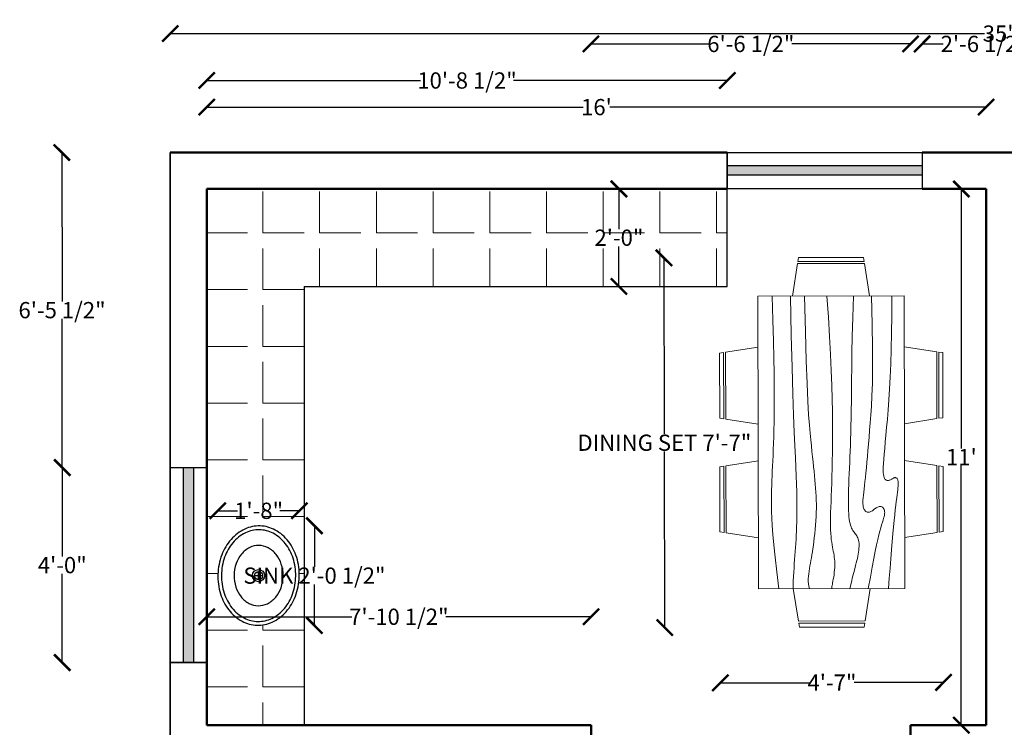
# Model space of a CAD drawing. Units: inches. Extents: x 2466 to 2986, y -30 to 527.
# Tile 3 of 5: x 2469 to 2711, y 353 to 527. Entities that reach past the tile are written whole.
import ezdxf

# ---------------------------------------------------------------- set-up
doc = ezdxf.new("R2010")
doc.units = ezdxf.units.IN
for name, color, linetype, lineweight in [('A-ANNO-DIMS', 2, 'Continuous', 18), ('A-FLOR-CASE', 32, 'Continuous', 25), ('A-FLOR-CASE-PATT', 5, 'Continuous', 13), ('A-FLOR-FIXT', 8, 'Continuous', 25), ('A-GLAZ', 4, 'Continuous', 25), ('A-GLAZ-PATT', 4, 'Continuous', 13), ('C-PROP', 40, 'Continuous', 35), ('furniture', 6, 'Continuous', 18), ('walls', 40, 'Continuous', 50)]:
    doc.layers.add(name, color=color, linetype=linetype, lineweight=lineweight)
doc.styles.get("Standard").update_dxf_attribs({"font": 'arial.ttf'})
doc.dimstyles.get("Standard").update_dxf_attribs({"dimtxt": 4, "dimasz": 4, "dimexe": 0.18, "dimexo": 0.0625, "dimgap": 0.09, "dimtad": 0, "dimtih": 1, "dimtoh": 1, "dimzin": 0, "dimdsep": 46, "dimlunit": 3, "dimtxsty": 'Standard', "dimblk": 'ARCHTICK', "dimcen": 0.09, "dimse1": 1, "dimse2": 1, "dimclrd": 3, "dimclrt": 2, "dimadec": 0, "dimazin": 0, "dimtfac": 1, "dimtofl": 0, "dimtmove": 0, "dimatfit": 3, "dimfxl": 1, "dimtolj": 1, "dimtzin": 0, "dimarcsym": 0})

# ---------------------------------------------------------------- blocks, each defined once
blk = doc.blocks.new('Dining Set - 36 x 72 in.')
for p, q in [((-22, 27.5), (-22.1562, 26.50042)), ((-22, 27.5), (-6, 27.5)), ((-5.8437, 26.49966), (-6, 27.5)), ((6, 27.5), (5.8438, 26.50042)), ((6, 27.5), (22, 27.5)), ((22.1563, 26.49966), (22, 27.5)), ((-22.2343, 26.00059), (-23.4847, 17.99762)), ((-22.2304, 26), (-5.7608, 26)), ((-5.8416, 26.5), (-22.1534, 26.5)), ((-4.5152, 17.99762), (-5.7655, 25.99926)), ((5.7657, 26.00059), (4.5153, 17.99762)), ((5.7696, 26), (22.2392, 26)), ((22.1584, 26.5), (5.8466, 26.5)), ((23.4848, 17.99762), (22.2345, 25.99926)), ((36, 18), (-36, 18)), ((-36, 18), (-36, -18)), ((36, -18), (36, 18)), ((-45.5, 8), (-44.5004, 8.15617)), ((-45.5, 8), (-45.5, -8)), ((-44.5, -8.15843), (-44.5, 8.15338)), ((-44.0006, 8.23428), (-35.9976, 9.48474)), ((-44, 8.23041), (-44, -8.23915)), ((44.0006, 8.23428), (35.9976, 9.48474)), ((44, 8.23041), (44, -8.23915)), ((44.5, -8.15843), (44.5, 8.15338)), ((45.5, 8), (44.5005, 8.15617)), ((45.5, 8), (45.5, -8)), ((-44.4997, -8.15631), (-45.5, -8)), ((-35.9976, -9.48476), (-43.9993, -8.2345)), ((35.9976, -9.48476), (43.9993, -8.2345)), ((44.4997, -8.15631), (45.5, -8)), ((-36, -18), (36, -18)), ((-22.2343, -26.0006), (-23.4847, -17.99762)), ((-4.5152, -17.99762), (-5.7655, -25.99928)), ((5.7657, -26.0006), (4.5153, -17.99762)), ((23.4848, -17.99762), (22.2345, -25.99928)), ((-22.2304, -26), (-5.7608, -26)), ((-22, -27.5), (-22.1562, -26.50044)), ((-5.8416, -26.5), (-22.1534, -26.5)), ((-5.8437, -26.49967), (-6, -27.5)), ((5.7696, -26), (22.2392, -26)), ((6, -27.5), (5.8438, -26.50044)), ((22.1584, -26.5), (5.8466, -26.5)), ((22.1563, -26.49967), (22, -27.5)), ((-22, -27.5), (-6, -27.5)), ((6, -27.5), (22, -27.5))]:
    blk.add_line(p, q)
for points in [[(-36, 15), (-31.1772, 14.97754), (-26.8079, 14.91406), (-22.8538, 14.81543), (-19.276, 14.6875), (-16.0362, 14.53613), (-13.0957, 14.36718), (-10.4159, 14.18652), (-7.9583, 14), (-5.6904, 13.81315), (-3.6035, 13.63021), (-1.6954, 13.45508), (0.0365, 13.29166), (1.5945, 13.14388), (2.9811, 13.01562), (4.1988, 12.9108), (5.25, 12.83333), (6.1393, 12.78613), (6.8802, 12.76823), (7.4883, 12.77767), (7.9792, 12.8125), (8.3685, 12.87077), (8.6719, 12.95052), (8.9049, 13.0498), (9.0833, 13.16666), (9.2205, 13.29899), (9.3216, 13.44401), (9.3895, 13.59879), (9.4271, 13.76041), (9.4373, 13.92594), (9.4232, 14.09245), (9.3875, 14.257), (9.3333, 14.41666), (9.2638, 14.56917), (9.1836, 14.71484), (9.0975, 14.85465), (9.0104, 14.98958), (8.9272, 15.1206), (8.8529, 15.2487), (8.7922, 15.37483), (8.75, 15.5), (8.7305, 15.62467), (8.7344, 15.74739), (8.7617, 15.86621), (8.8125, 15.97916), (8.8867, 16.08431), (8.9844, 16.17968), (9.1055, 16.26334), (9.25, 16.33333), (9.4189, 16.38802), (9.6172, 16.42708), (9.8506, 16.45052), (10.125, 16.45833), (10.4463, 16.45052), (10.8203, 16.42708), (11.2529, 16.38802), (11.75, 16.33333), (12.3184, 16.26318), (12.9694, 16.17838), (13.7151, 16.07991), (14.5677, 15.96875), (15.5395, 15.84586), (16.6426, 15.71224), (17.8893, 15.56884), (19.2917, 15.41666), (20.859, 15.25667), (22.5879, 15.08984), (24.4721, 14.91715), (26.5052, 14.73958), (28.6809, 14.5581), (30.9929, 14.3737), (33.4347, 14.18733), (36, 14)], [(-36, 10), (-28.9766, 10.14274), (-23.1725, 10.20442), (-18.4241, 10.19775), (-14.5677, 10.13541), (-11.4399, 10.03011), (-8.877, 9.89453), (-6.7154, 9.74137), (-4.7917, 9.58333), (-2.9698, 9.43082), (-1.2246, 9.28515), (0.4415, 9.14534), (2.026, 9.01041), (3.5266, 8.87939), (4.9408, 8.7513), (6.266, 8.62516), (7.5, 8.5), (8.6411, 8.37549), (9.6914, 8.2539), (10.6538, 8.13818), (11.5312, 8.03125), (12.3267, 7.93603), (13.043, 7.85547), (13.6831, 7.79248), (14.25, 7.75), (14.7471, 7.7303), (15.1797, 7.73307), (15.5537, 7.75732), (15.875, 7.80208), (16.1494, 7.86637), (16.3828, 7.94922), (16.5811, 8.04964), (16.75, 8.16666), (16.8944, 8.29915), (17.0143, 8.44531), (17.1089, 8.60319), (17.1771, 8.77083), (17.218, 8.94629), (17.2305, 9.1276), (17.2137, 9.31282), (17.1667, 9.5), (17.0895, 9.6875), (16.987, 9.875), (16.8649, 10.0625), (16.7292, 10.25), (16.5856, 10.4375), (16.4401, 10.625), (16.2985, 10.8125), (16.1667, 11), (16.05, 11.18733), (15.9518, 11.3737), (15.8752, 11.5581), (15.8229, 11.73958), (15.798, 11.91715), (15.8034, 12.08984), (15.842, 12.25667), (15.9167, 12.41666), (16.0295, 12.56836), (16.1784, 12.70833), (16.3605, 12.83268), (16.5729, 12.9375), (16.8127, 13.01888), (17.0768, 13.07291), (17.3625, 13.0957), (17.6667, 13.08333), (17.9894, 13.03312), (18.3418, 12.94726), (18.7382, 12.82918), (19.1927, 12.68229), (19.7195, 12.51001), (20.3327, 12.31575), (21.0465, 12.10294), (21.875, 11.875), (22.8357, 11.63354), (23.959, 11.37304), (25.2786, 11.08618), (26.8282, 10.76562), (28.6414, 10.40405), (30.752, 9.99414), (33.1936, 9.52856), (36, 9)], [(-36, 5.5), (-30.7157, 5.3348), (-26.069, 5.20963), (-21.9946, 5.11767), (-18.4271, 5.05208), (-15.3009, 5.00602), (-12.5508, 4.97265), (-10.1112, 4.94515), (-7.9167, 4.91666), (-5.909, 4.88167), (-4.0586, 4.83984), (-2.3429, 4.79215), (-0.7396, 4.73958), (0.7739, 4.6831), (2.22, 4.6237), (3.6213, 4.56233), (5, 4.5), (6.373, 4.43782), (7.7344, 4.3776), (9.0723, 4.32129), (10.375, 4.27083), (11.6309, 4.22819), (12.8281, 4.19531), (13.9551, 4.17415), (15, 4.16666), (15.954, 4.17448), (16.819, 4.19791), (17.6001, 4.23698), (18.3021, 4.29166), (18.9299, 4.36198), (19.4883, 4.44791), (19.9823, 4.54948), (20.4167, 4.66666), (20.7969, 4.79899), (21.1302, 4.94401), (21.4245, 5.09879), (21.6875, 5.26041), (21.9271, 5.42594), (22.1511, 5.59245), (22.3672, 5.757), (22.5834, 5.91666), (22.8065, 6.06868), (23.0404, 6.21093), (23.2879, 6.34147), (23.5521, 6.45833), (23.8358, 6.55957), (24.142, 6.64323), (24.4735, 6.70735), (24.8334, 6.75), (25.2235, 6.76969), (25.642, 6.76692), (26.0858, 6.74267), (26.5521, 6.69791), (27.0379, 6.63362), (27.5404, 6.55078), (28.0565, 6.45036), (28.5834, 6.33333), (29.1242, 6.19987), (29.7071, 6.04687), (30.3661, 5.87044), (31.1354, 5.66666), (32.0493, 5.43164), (33.142, 5.16146), (34.4475, 4.85221), (36, 4.5)], [(-36, -1), (-30.7915, -0.6591), (-26.0195, -0.38216), (-21.6519, -0.16284), (-17.6563, 0.00521), (-14.0005, 0.12833), (-10.6523, 0.21289), (-7.5796, 0.26522), (-4.75, 0.29166), (-2.134, 0.29793), (0.2878, 0.28711), (2.5317, 0.26163), (4.6146, 0.22396), (6.5529, 0.17651), (8.3633, 0.12174), (10.0623, 0.06209), (11.6667, 0), (13.1899, -0.06201), (14.6341, -0.1211), (15.9982, -0.17432), (17.2813, -0.21875), (18.4823, -0.25147), (19.6003, -0.26953), (20.6343, -0.27002), (21.5834, -0.25), (22.4481, -0.20768), (23.2357, -0.14584), (23.9549, -0.06836), (24.6146, 0.02083), (25.2235, 0.11784), (25.7904, 0.21875), (26.3241, 0.31966), (26.8334, 0.41666), (27.3265, 0.50618), (27.8099, 0.58593), (28.2894, 0.65397), (28.7709, 0.70833), (29.2601, 0.74707), (29.763, 0.76823), (30.2855, 0.76985), (30.8334, 0.75), (31.4088, 0.70784), (31.9994, 0.64713), (32.589, 0.57275), (33.1615, 0.48958), (33.7008, 0.4025), (34.1908, 0.3164), (34.6153, 0.23616), (34.9584, 0.16666), (35.2099, 0.11165), (35.3848, 0.07031), (35.504, 0.04069), (35.5886, 0.02083), (35.6594, 0.00879), (35.7377, 0.0026), (35.8442, 0.00032), (36, 0)], [(-36, -6.5), (-27.1843, -6.31267), (-20.084, -6.1263), (-14.469, -5.9419), (-10.1094, -5.76042), (-6.7752, -5.58285), (-4.2363, -5.41016), (-2.2629, -5.24333), (-0.625, -5.08334), (0.8708, -4.93099), (2.2715, -4.78646), (3.5872, -4.64974), (4.8281, -4.52084), (6.0046, -4.39974), (7.127, -4.28646), (8.2053, -4.18099), (9.25, -4.08334), (10.2705, -3.99382), (11.2734, -3.91407), (12.2647, -3.84603), (13.25, -3.79167), (14.2354, -3.75293), (15.2266, -3.73177), (16.2295, -3.73015), (17.25, -3.75), (18.2912, -3.79248), (19.3451, -3.85547), (20.4009, -3.93604), (21.4479, -4.03125), (22.4754, -4.13819), (23.4727, -4.25391), (24.4289, -4.37549), (25.3334, -4.5), (26.1785, -4.62492), (26.9694, -4.74935), (27.7145, -4.87281), (28.4219, -4.99479), (29.1, -5.11483), (29.7572, -5.23242), (30.4016, -5.34709), (31.0417, -5.45834), (31.6837, -5.56437), (32.3262, -5.65821), (32.9658, -5.73153), (33.599, -5.77604), (34.2224, -5.78345), (34.8327, -5.74545), (35.4264, -5.65373), (36, -5.5)], [(-36, -10), (-26.4022, -9.81299), (-18.4675, -9.62891), (-11.9839, -9.45069), (-6.7396, -9.28125), (-2.5226, -9.12354), (0.8789, -8.98047), (3.6769, -8.85498), (6.0833, -8.75), (8.2767, -8.66765), (10.3021, -8.60677), (12.1712, -8.56543), (13.8958, -8.54167), (15.4876, -8.53353), (16.9583, -8.53907), (18.3197, -8.55632), (19.5834, -8.58334), (20.7616, -8.61841), (21.8685, -8.66081), (22.9188, -8.71004), (23.9271, -8.76563), (24.9081, -8.82707), (25.8763, -8.89388), (26.8465, -8.96558), (27.8334, -9.04167), (28.8474, -9.12118), (29.8828, -9.20117), (30.93, -9.27824), (31.9792, -9.34896), (33.0205, -9.40991), (34.0443, -9.45768), (35.0407, -9.48885), (36, -9.5)], [(-36, -14.5), (-30.0881, -14.33513), (-25.0332, -14.21224), (-20.7312, -14.12647), (-17.0781, -14.07292), (-13.97, -14.04671), (-11.3027, -14.04297), (-8.9724, -14.05681), (-6.875, -14.08334), (-4.9224, -14.11833), (-3.0905, -14.16016), (-1.3709, -14.20785), (0.2448, -14.26042), (1.7647, -14.3169), (3.1973, -14.3763), (4.5507, -14.43767), (5.8333, -14.5), (7.0554, -14.5621), (8.235, -14.62175), (9.3922, -14.67652), (10.5469, -14.72396), (11.7192, -14.76164), (12.929, -14.78711), (14.1965, -14.79794), (15.5417, -14.79167), (16.9933, -14.76424), (18.6152, -14.70508), (20.4804, -14.60197), (22.6615, -14.44271), (25.2312, -14.21509), (28.2624, -13.9069), (31.8277, -13.50594), (36, -13)]]:
    blk.add_lwpolyline(points)
blk = doc.blocks.new('Sink - Oval top')
for p, q in [((-1, 0), (1, 0)), ((0, 1), (0, -1))]:
    blk.add_line(p, q)
for points in [[(-12.23, 0.39, 0.117634), (-11.46, -3.36, 0.104469), (-8.88, -6.8, 0.090016), (-5.08, -9.07, 0.08192), (-0.32, -10.02, 0.08192), (4.49, -9.38, 0.090016), (8.42, -7.36, 0.104469), (11.22, -4.09, 0.117634), (12.23, -0.39, 0.117634), (11.46, 3.36, 0.104469), (8.88, 6.8, 0.090016), (5.08, 9.07, 0.08192), (0.32, 10.02, 0.08192), (-4.49, 9.38, 0.090016), (-8.42, 7.36, 0.104469), (-11.22, 4.09, 0.117634)], [(-11.29, 0.16, 0.118622), (-10.52, -3.25, 0.104678), (-8.07, -6.36, 0.089562), (-4.54, -8.37, 0.081185), (-0.13, -9.15, 0.081185), (4.3, -8.49, 0.089562), (7.89, -6.58, 0.104678), (10.42, -3.55, 0.118622), (11.29, -0.16, 0.118622), (10.52, 3.25, 0.104678), (8.07, 6.36, 0.089562), (4.54, 8.37, 0.081185), (0.13, 9.15, 0.081185), (-4.3, 8.49, 0.089562), (-7.89, 6.58, 0.104678), (-10.42, 3.55, 0.118622)], [(-7.42, 0.08, 0.118283), (-6.91, -2.17, 0.104607), (-5.29, -4.21, 0.089718), (-2.97, -5.53, 0.081436), (-0.07, -6.04, 0.081436), (2.84, -5.59, 0.089718), (5.2, -4.33, 0.104607), (6.86, -2.32, 0.118283), (7.42, -0.08, 0.118283), (6.91, 2.17, 0.104607), (5.29, 4.21, 0.089718), (2.97, 5.53, 0.081436), (0.07, 6.04, 0.081436), (-2.84, 5.59, 0.089718), (-5.2, 4.33, 0.104607), (-6.86, 2.32, 0.118283)]]:
    blk.add_lwpolyline(points, format="xyb", close=True)
for radius in [1.5, 1]:
    blk.add_circle((0, 0), radius)
blk = doc.blocks.new('_ArchTick')
at = {"color": 0, "linetype": 'ByBlock', "const_width": 0.15}
blk.add_lwpolyline([(-0.5, -0.5), (0.5, 0.5)], dxfattribs=at)
blk = doc.blocks.new('*D21')
at = {"layer": 'A-ANNO-DIMS', "color": 0, "lineweight": -2, "transparency": 16777216}
for p, q in [((2505.73, 524.05), (2706.38, 524.05)), ((2928.73, 524.05), (2728.07, 524.05))]:
    blk.add_line(p, q, dxfattribs=at)
at = {"layer": 'Defpoints', "color": 0, "transparency": 16777216}
for p in [(2928.73, 524.05), (2505.73, 494.8), (2928.73, 494.8)]:
    blk.add_point(p, dxfattribs=at)
at = {"layer": 'A-ANNO-DIMS', "color": 0, "lineweight": -2, "transparency": 16777216, "xscale": 4, "yscale": 4, "zscale": 4, "rotation": 180}
blk.add_blockref('_ArchTick', (2505.73, 524.05), dxfattribs=at)
at = {"layer": 'A-ANNO-DIMS', "color": 0, "lineweight": -2, "transparency": 16777216, "xscale": 4, "yscale": 4, "zscale": 4}
blk.add_blockref('_ArchTick', (2928.73, 524.05), dxfattribs=at)
at = {"layer": 'A-ANNO-DIMS', "color": 0, "transparency": 16777216, "insert": (2717.23, 524.05), "char_height": 4, "attachment_point": 5}
blk.add_mtext('\\A1;35\'-3.00"', dxfattribs=at)
blk = doc.blocks.new('*D23')
at = {"layer": 'A-ANNO-DIMS', "color": 0, "lineweight": -2, "transparency": 16777216}
for p, q in [((2514.73, 505.95), (2607.43, 505.95)), ((2706.73, 505.95), (2614.02, 505.95))]:
    blk.add_line(p, q, dxfattribs=at)
at = {"layer": 'Defpoints', "color": 0, "transparency": 16777216}
for p in [(2706.73, 505.95), (2514.73, 485.8), (2706.73, 485.8)]:
    blk.add_point(p, dxfattribs=at)
at = {"layer": 'A-ANNO-DIMS', "color": 0, "lineweight": -2, "transparency": 16777216, "xscale": 4, "yscale": 4, "zscale": 4, "rotation": 180}
blk.add_blockref('_ArchTick', (2514.73, 505.95), dxfattribs=at)
at = {"layer": 'A-ANNO-DIMS', "color": 0, "lineweight": -2, "transparency": 16777216, "xscale": 4, "yscale": 4, "zscale": 4}
blk.add_blockref('_ArchTick', (2706.73, 505.95), dxfattribs=at)
at = {"layer": 'A-ANNO-DIMS', "color": 0, "transparency": 16777216, "insert": (2610.73, 505.95), "char_height": 4, "attachment_point": 5}
blk.add_mtext("\\A1;16'", dxfattribs=at)
blk = doc.blocks.new('*D25')
at = {"layer": 'A-ANNO-DIMS', "color": 0, "lineweight": -2, "transparency": 16777216}
for p, q in [((2700.63, 485.8), (2700.63, 421.89)), ((2700.63, 353.8), (2700.63, 417.7))]:
    blk.add_line(p, q, dxfattribs=at)
at = {"layer": 'Defpoints', "color": 0, "transparency": 16777216}
for p in [(2706.73, 485.8), (2700.63, 353.8), (2706.73, 353.8)]:
    blk.add_point(p, dxfattribs=at)
at = {"layer": 'A-ANNO-DIMS', "color": 0, "lineweight": -2, "transparency": 16777216, "xscale": 4, "yscale": 4, "zscale": 4}
for p, rotation in [((2700.63, 485.8), 90), ((2700.63, 353.8), 270)]:
    blk.add_blockref('_ArchTick', p, dxfattribs=dict(at, rotation=rotation))
at = {"layer": 'A-ANNO-DIMS', "color": 0, "transparency": 16777216, "insert": (2700.63, 419.8), "char_height": 4, "attachment_point": 5}
blk.add_mtext("\\A1;11'", dxfattribs=at)
blk = doc.blocks.new('WIN-48IN')
h = blk.add_hatch(color=256)
h.dxf.hatch_style = 1
h.paths.add_polyline_path([(0, 5.81), (0, 3.39), (48, 3.39), (48, 5.81)])
for p, q in [((0, 9), (0, 0)), ((48, 9), (48, 0))]:
    blk.add_line(p, q)
for points in [[(0, 9), (48, 9), (48, 0), (0, 0)], [(0, 5.81), (48, 5.81), (48, 3.39), (0, 3.39)]]:
    blk.add_lwpolyline(points, close=True)
blk = doc.blocks.new('*D53')
at = {"layer": 'A-ANNO-DIMS', "color": 3, "lineweight": -2, "transparency": 16777216}
for p, q in [((2627.36, 468.84), (2627.46, 425.5)), ((2627.58, 377.84), (2627.47, 421.18))]:
    blk.add_line(p, q, dxfattribs=at)
at = {"layer": 'Defpoints', "color": 0, "transparency": 16777216}
for p in [(2641.01, 468.87), (2627.58, 377.84), (2641.23, 377.87)]:
    blk.add_point(p, dxfattribs=at)
at = {"layer": 'A-ANNO-DIMS', "color": 3, "lineweight": -2, "transparency": 16777216, "xscale": 4, "yscale": 4, "zscale": 4}
for p, rotation in [((2627.36, 468.84), 90.1373256303258), ((2627.58, 377.84), 270.1373256303258)]:
    blk.add_blockref('_ArchTick', p, dxfattribs=dict(at, rotation=rotation))
at = {"layer": 'A-ANNO-DIMS', "color": 2, "transparency": 16777216, "insert": (2627.47, 423.34), "char_height": 4, "attachment_point": 5}
blk.add_mtext('\\A1;DINING SET 7\'-7"', dxfattribs=at)
blk = doc.blocks.new('*D54')
at = {"layer": 'A-ANNO-DIMS', "color": 3, "lineweight": -2, "transparency": 16777216}
for p, q in [((2641.26, 364.22), (2663.27, 364.27)), ((2696.26, 364.35), (2674.25, 364.3))]:
    blk.add_line(p, q, dxfattribs=at)
at = {"layer": 'Defpoints', "color": 0, "transparency": 16777216}
for p in [(2641.23, 377.87), (2696.23, 378), (2696.26, 364.35)]:
    blk.add_point(p, dxfattribs=at)
at = {"layer": 'A-ANNO-DIMS', "color": 3, "lineweight": -2, "transparency": 16777216, "xscale": 4, "yscale": 4, "zscale": 4}
for p, rotation in [((2641.26, 364.22), 180.1373256303259), ((2696.26, 364.35), 0.1373256303258501)]:
    blk.add_blockref('_ArchTick', p, dxfattribs=dict(at, rotation=rotation))
at = {"layer": 'A-ANNO-DIMS', "color": 2, "transparency": 16777216, "insert": (2668.76, 364.29), "char_height": 4, "attachment_point": 5}
blk.add_mtext('\\A1;4\'-7"', dxfattribs=at)
blk = doc.blocks.new('*D59')
at = {"layer": 'A-ANNO-DIMS', "color": 3, "lineweight": -2, "transparency": 16777216}
for p, q in [((2541.26, 402.9), (2541.26, 392.78)), ((2541.26, 378.35), (2541.26, 388.46))]:
    blk.add_line(p, q, dxfattribs=at)
at = {"layer": 'Defpoints', "color": 0, "transparency": 16777216}
for p in [(2537.57, 402.9), (2541.26, 402.9), (2537.57, 378.35)]:
    blk.add_point(p, dxfattribs=at)
at = {"layer": 'A-ANNO-DIMS', "color": 3, "lineweight": -2, "transparency": 16777216, "xscale": 4, "yscale": 4, "zscale": 4}
for p, rotation in [((2541.26, 402.9), 90), ((2541.26, 378.35), 270)]:
    blk.add_blockref('_ArchTick', p, dxfattribs=dict(at, rotation=rotation))
at = {"layer": 'A-ANNO-DIMS', "color": 2, "transparency": 16777216, "insert": (2541.26, 390.62), "char_height": 4, "attachment_point": 5}
blk.add_mtext('\\A1;SINK 2\'-0 1/2"', dxfattribs=at)
blk = doc.blocks.new('*D60')
at = {"layer": 'A-ANNO-DIMS', "color": 3, "lineweight": -2, "transparency": 16777216}
for p, q in [((2517.44, 406.58), (2522.29, 406.58)), ((2537.57, 406.58), (2532.72, 406.58))]:
    blk.add_line(p, q, dxfattribs=at)
at = {"layer": 'Defpoints', "color": 0, "transparency": 16777216}
for p in [(2517.44, 406.58), (2517.44, 402.9), (2537.57, 402.9)]:
    blk.add_point(p, dxfattribs=at)
at = {"layer": 'A-ANNO-DIMS', "color": 3, "lineweight": -2, "transparency": 16777216, "xscale": 4, "yscale": 4, "zscale": 4, "rotation": 180}
blk.add_blockref('_ArchTick', (2517.44, 406.58), dxfattribs=at)
at = {"layer": 'A-ANNO-DIMS', "color": 3, "lineweight": -2, "transparency": 16777216, "xscale": 4, "yscale": 4, "zscale": 4}
blk.add_blockref('_ArchTick', (2537.57, 406.58), dxfattribs=at)
at = {"layer": 'A-ANNO-DIMS', "color": 2, "transparency": 16777216, "insert": (2527.51, 406.58), "char_height": 4, "attachment_point": 5}
blk.add_mtext('\\A1;1\'-8"', dxfattribs=at)
blk = doc.blocks.new('*D62')
at = {"layer": 'A-ANNO-DIMS', "color": 3, "lineweight": -2, "transparency": 16777216}
for p, q in [((2609.4, 521.5), (2638.69, 521.5)), ((2688.14, 521.5), (2658.85, 521.5))]:
    blk.add_line(p, q, dxfattribs=at)
at = {"layer": 'Defpoints', "color": 0, "transparency": 16777216}
for p in [(2688.14, 521.5), (2609.4, 353.8), (2688.14, 353.8)]:
    blk.add_point(p, dxfattribs=at)
at = {"layer": 'A-ANNO-DIMS', "color": 3, "lineweight": -2, "transparency": 16777216, "xscale": 4, "yscale": 4, "zscale": 4, "rotation": 180}
blk.add_blockref('_ArchTick', (2609.4, 521.5), dxfattribs=at)
at = {"layer": 'A-ANNO-DIMS', "color": 3, "lineweight": -2, "transparency": 16777216, "xscale": 4, "yscale": 4, "zscale": 4}
blk.add_blockref('_ArchTick', (2688.14, 521.5), dxfattribs=at)
at = {"layer": 'A-ANNO-DIMS', "color": 2, "transparency": 16777216, "insert": (2648.77, 521.5), "char_height": 4, "attachment_point": 5}
blk.add_mtext('\\A1;6\'-6 1/2"', dxfattribs=at)
blk = doc.blocks.new('*D69')
at = {"layer": 'A-ANNO-DIMS', "color": 3, "lineweight": -2, "transparency": 16777216}
for p, q in [((2616.28, 485.8), (2616.28, 475.93)), ((2616.28, 461.8), (2616.28, 471.66))]:
    blk.add_line(p, q, dxfattribs=at)
at = {"layer": 'Defpoints', "color": 0, "transparency": 16777216}
for p in [(2616.28, 485.8), (2642.98, 485.8), (2642.98, 461.8)]:
    blk.add_point(p, dxfattribs=at)
at = {"layer": 'A-ANNO-DIMS', "color": 3, "lineweight": -2, "transparency": 16777216, "xscale": 4, "yscale": 4, "zscale": 4}
for p, rotation in [((2616.28, 485.8), 90), ((2616.28, 461.8), 270)]:
    blk.add_blockref('_ArchTick', p, dxfattribs=dict(at, rotation=rotation))
at = {"layer": 'A-ANNO-DIMS', "color": 2, "transparency": 16777216, "insert": (2616.28, 473.8), "char_height": 4, "attachment_point": 5}
blk.add_mtext('\\A1;2\'-0"', dxfattribs=at)
blk = doc.blocks.new('*D72')
at = {"layer": 'A-ANNO-DIMS', "color": 3, "lineweight": -2, "transparency": 16777216}
for p, q in [((2514.73, 512.5), (2567.42, 512.5)), ((2642.98, 512.5), (2590.28, 512.5))]:
    blk.add_line(p, q, dxfattribs=at)
at = {"layer": 'Defpoints', "color": 0, "transparency": 16777216}
for p in [(2642.98, 512.5), (2514.73, 485.8), (2642.98, 485.8)]:
    blk.add_point(p, dxfattribs=at)
at = {"layer": 'A-ANNO-DIMS', "color": 3, "lineweight": -2, "transparency": 16777216, "xscale": 4, "yscale": 4, "zscale": 4, "rotation": 180}
blk.add_blockref('_ArchTick', (2514.73, 512.5), dxfattribs=at)
at = {"layer": 'A-ANNO-DIMS', "color": 3, "lineweight": -2, "transparency": 16777216, "xscale": 4, "yscale": 4, "zscale": 4}
blk.add_blockref('_ArchTick', (2642.98, 512.5), dxfattribs=at)
at = {"layer": 'A-ANNO-DIMS', "color": 2, "transparency": 16777216, "insert": (2578.85, 512.5), "char_height": 4, "attachment_point": 5}
blk.add_mtext('\\A1;10\'-8 1/2"', dxfattribs=at)
blk = doc.blocks.new('*D73')
at = {"layer": 'A-ANNO-DIMS', "color": 3, "lineweight": -2, "transparency": 16777216}
for p, q in [((2690.98, 521.5), (2696.18, 521.5)), ((2721.59, 521.5), (2716.38, 521.5))]:
    blk.add_line(p, q, dxfattribs=at)
at = {"layer": 'Defpoints', "color": 0, "transparency": 16777216}
for p in [(2721.59, 521.5), (2690.98, 494.8), (2721.59, 494.8)]:
    blk.add_point(p, dxfattribs=at)
at = {"layer": 'A-ANNO-DIMS', "color": 3, "lineweight": -2, "transparency": 16777216, "xscale": 4, "yscale": 4, "zscale": 4, "rotation": 180}
blk.add_blockref('_ArchTick', (2690.98, 521.5), dxfattribs=at)
at = {"layer": 'A-ANNO-DIMS', "color": 3, "lineweight": -2, "transparency": 16777216, "xscale": 4, "yscale": 4, "zscale": 4}
blk.add_blockref('_ArchTick', (2721.59, 521.5), dxfattribs=at)
at = {"layer": 'A-ANNO-DIMS', "color": 2, "transparency": 16777216, "insert": (2706.28, 521.5), "char_height": 4, "attachment_point": 5}
blk.add_mtext('\\A1;2\'-6 1/2"', dxfattribs=at)
blk = doc.blocks.new('*D74')
at = {"layer": 'A-ANNO-DIMS', "color": 3, "lineweight": -2, "transparency": 16777216}
for p, q in [((2479.03, 494.76), (2479.07, 458.13)), ((2479.13, 417.18), (2479.08, 453.81))]:
    blk.add_line(p, q, dxfattribs=at)
at = {"layer": 'Defpoints', "color": 0, "transparency": 16777216}
for p in [(2479.03, 494.76), (2505.73, 494.8), (2505.83, 417.21)]:
    blk.add_point(p, dxfattribs=at)
at = {"layer": 'A-ANNO-DIMS', "color": 3, "lineweight": -2, "transparency": 16777216, "xscale": 4, "yscale": 4, "zscale": 4}
for p, rotation in [((2479.03, 494.76), 90.07540096896105), ((2479.13, 417.18), 270.075400968961)]:
    blk.add_blockref('_ArchTick', p, dxfattribs=dict(at, rotation=rotation))
at = {"layer": 'A-ANNO-DIMS', "color": 2, "transparency": 16777216, "insert": (2479.08, 455.97), "char_height": 4, "attachment_point": 5}
blk.add_mtext('\\A1;6\'-5 1/2"', dxfattribs=at)
blk = doc.blocks.new('*D82')
at = {"layer": 'A-ANNO-DIMS', "color": 3, "lineweight": -2, "transparency": 16777216}
for p, q in [((2479.13, 417.21), (2479.13, 395.34)), ((2479.13, 369.21), (2479.13, 391.08))]:
    blk.add_line(p, q, dxfattribs=at)
at = {"layer": 'Defpoints', "color": 0, "transparency": 16777216}
for p in [(2479.13, 417.21), (2505.83, 417.21), (2505.83, 369.21)]:
    blk.add_point(p, dxfattribs=at)
at = {"layer": 'A-ANNO-DIMS', "color": 3, "lineweight": -2, "transparency": 16777216, "xscale": 4, "yscale": 4, "zscale": 4}
for p, rotation in [((2479.13, 417.21), 90), ((2479.13, 369.21), 270)]:
    blk.add_blockref('_ArchTick', p, dxfattribs=dict(at, rotation=rotation))
at = {"layer": 'A-ANNO-DIMS', "color": 2, "transparency": 16777216, "insert": (2479.13, 393.21), "char_height": 4, "attachment_point": 5}
blk.add_mtext('\\A1;4\'-0"', dxfattribs=at)
blk = doc.blocks.new('*D84')
at = {"layer": 'A-ANNO-DIMS', "color": 3, "lineweight": -2, "transparency": 16777216}
for p, q in [((2514.73, 380.5), (2550.46, 380.5)), ((2609.4, 380.5), (2573.67, 380.5))]:
    blk.add_line(p, q, dxfattribs=at)
at = {"layer": 'Defpoints', "color": 0, "transparency": 16777216}
for p in [(2609.4, 380.5), (2514.73, 353.8), (2609.4, 353.8)]:
    blk.add_point(p, dxfattribs=at)
at = {"layer": 'A-ANNO-DIMS', "color": 3, "lineweight": -2, "transparency": 16777216, "xscale": 4, "yscale": 4, "zscale": 4, "rotation": 180}
blk.add_blockref('_ArchTick', (2514.73, 380.5), dxfattribs=at)
at = {"layer": 'A-ANNO-DIMS', "color": 3, "lineweight": -2, "transparency": 16777216, "xscale": 4, "yscale": 4, "zscale": 4}
blk.add_blockref('_ArchTick', (2609.4, 380.5), dxfattribs=at)
at = {"layer": 'A-ANNO-DIMS', "color": 2, "transparency": 16777216, "insert": (2562.06, 380.5), "char_height": 4, "attachment_point": 5}
blk.add_mtext('\\A1;7\'-10 1/2"', dxfattribs=at)

msp = doc.modelspace()

# ---------------------------------------------------------------- hatches: boundary and pattern name
at = {"layer": 'A-FLOR-CASE-PATT'}
h = msp.add_hatch(dxfattribs=at)
h.set_pattern_fill('ANGLE', color=256, scale=2)
h.set_pattern_definition([(0, (0, 0), (0, 13.97), [10.16, -3.81]), (90, (0, 0), (-13.97, 9e-16), [10.16, -3.81])])
h.paths.add_polyline_path([(2642.976, 485.795), (2514.725, 485.795), (2514.725, 417.211), (2514.828, 417.211), (2514.828, 369.211), (2514.725, 353.795), (2538.725, 353.795), (2538.725, 461.795), (2642.976, 461.795)])
h.paths.add_polyline_path([(2527.9, 402.857, -0.1176343), (2531.599, 401.847, -0.1044693), (2534.867, 399.045, -0.0900158), (2536.886, 395.111, -0.0819199), (2537.521, 390.3, -0.0819199), (2536.578, 385.54, -0.0900158), (2534.309, 381.744, -0.1044693), (2530.867, 379.158, -0.1176343), (2527.111, 378.389, -0.1176343), (2523.413, 379.398, -0.1044693), (2520.145, 382.2, -0.0900158), (2518.125, 386.135, -0.0819199), (2517.49, 390.946, -0.0819199), (2518.433, 395.706, -0.0900158), (2520.702, 399.502, -0.1044693), (2524.144, 402.087, -0.1176343)], flags=16)
h.paths.add_polyline_path([(2527.665, 401.909, -0.1186217), (2531.054, 401.043, -0.1046782), (2534.089, 398.512, -0.0895621), (2535.997, 394.923, -0.0811847), (2536.657, 390.494, -0.0811847), (2535.873, 386.085, -0.0895621), (2533.864, 382.551, -0.1046782), (2530.759, 380.107, -0.1186217), (2527.346, 379.337, -0.1186217), (2523.957, 380.203, -0.1046782), (2520.922, 382.733, -0.0895621), (2519.014, 386.323, -0.0811847), (2518.354, 390.752, -0.0811847), (2519.139, 395.161, -0.0895621), (2521.147, 398.695, -0.1046782), (2524.252, 401.139, -0.1186217)], flags=0)
h.paths.add_polyline_path([(2527.589, 398.043, -0.1182826), (2529.827, 397.48, -0.1046075), (2531.833, 395.822, -0.089718), (2533.099, 393.465, -0.0814361), (2533.542, 390.555, -0.0814361), (2533.034, 387.656, -0.089718), (2531.716, 385.328, -0.1046075), (2529.673, 383.716, -0.1182826), (2527.423, 383.202, -0.1182826), (2525.184, 383.766, -0.1046075), (2523.178, 385.423, -0.089718), (2521.912, 387.781, -0.0814361), (2521.469, 390.69, -0.0814361), (2521.977, 393.589, -0.089718), (2523.296, 395.918, -0.1046075), (2525.338, 397.53, -0.1182826)], flags=0)
h.paths.add_polyline_path([(2526.506, 390.623, -1), (2528.506, 390.623, -1)], flags=0)
at = {"layer": 'A-GLAZ-PATT'}
h = msp.add_hatch(color=256, dxfattribs=at)
h.dxf.hatch_style = 1
h.paths.add_polyline_path([(2509.018, 369.211), (2511.433, 369.211), (2511.433, 417.211), (2509.018, 417.211)])

# ---------------------------------------------------------------- linework, layer by layer
at = {"layer": 'A-FLOR-CASE'}
for p, q in [((2642.976, 461.795), (2642.976, 485.795)), ((2538.725, 461.795), (2538.725, 353.795)), ((2538.725, 461.795), (2642.976, 461.795))]:
    msp.add_line(p, q, dxfattribs=at)
at = {"layer": 'A-GLAZ'}
for p, q in [((2505.828, 417.211), (2514.828, 417.211)), ((2505.828, 369.211), (2514.828, 369.211))]:
    msp.add_line(p, q, dxfattribs=at)
for points in [[(2505.828, 369.211), (2505.828, 417.211), (2514.828, 417.211), (2514.828, 369.211)], [(2509.018, 369.211), (2509.018, 417.211), (2511.433, 417.211), (2511.433, 369.211)]]:
    msp.add_lwpolyline(points, close=True, dxfattribs=at)
at = {"layer": 'C-PROP'}
msp.add_line((2505.725, 494.795), (2505.725, -0.205), dxfattribs=at)
at = {"layer": 'walls'}
for p, q in [((2505.725, 494.795), (2642.976, 494.795)), ((2690.976, 494.795), (2928.725, 494.795)), ((2514.725, 485.795), (2642.976, 485.795)), ((2514.725, 485.795), (2514.725, 353.795)), ((2690.976, 485.795), (2706.725, 485.795)), ((2706.725, 485.795), (2706.725, 353.795)), ((2514.725, 353.795), (2609.399, 353.795)), ((2609.399, 353.795), (2609.399, 344.795)), ((2688.139, 353.795), (2706.725, 353.795)), ((2688.139, 353.795), (2688.139, 344.795))]:
    msp.add_line(p, q, dxfattribs=at)

# ---------------------------------------------------------------- block references
at = {"layer": 'A-FLOR-FIXT', "rotation": 90.00000000000003}
msp.add_blockref('Sink - Oval top', (2527.506, 390.623), dxfattribs=at)
at = {"layer": 'A-GLAZ'}
msp.add_blockref('WIN-48IN', (2642.976, 485.795), dxfattribs=at)
at = {"layer": 'furniture', "rotation": 270.1373256303258}
msp.add_blockref('Dining Set - 36 x 72 in.', (2668.618, 423.438), dxfattribs=at)

# ---------------------------------------------------------------- dimensions: what is measured, and where the dimension line sits
at = {"layer": 'A-ANNO-DIMS'}
for base, p1, p2, override, picture, middle in [((2928.725, 524.047), (2505.725, 494.795), (2928.725, 494.795), {"dimclrd": 0, "dimclre": 0, "dimclrt": 0}, '*D21', (2717.225, 524.047)), ((2688.139, 521.495), (2609.399, 353.795), (2688.139, 353.795), {"dimdec": 1, "dimlfac": 1, "dimrnd": 0, "dimzin": 1, "dimdsep": 46, "dimlunit": 4, "dimfrac": 2}, '*D62', (2648.769, 521.495)), ((2721.59, 521.495), (2690.976, 494.795), (2721.59, 494.795), {"dimdec": 1, "dimlfac": 1, "dimrnd": 0, "dimzin": 1, "dimdsep": 46, "dimlunit": 4, "dimfrac": 2}, '*D73', (2706.283, 521.495)), ((2706.725, 505.95), (2514.725, 485.795), (2706.725, 485.795), {"dimclrd": 0, "dimclre": 0, "dimclrt": 0}, '*D23', (2610.725, 505.95)), ((2609.399, 380.495), (2514.725, 353.795), (2609.399, 353.795), {"dimdec": 1, "dimlfac": 1, "dimrnd": 0, "dimzin": 1, "dimdsep": 46, "dimlunit": 4, "dimfrac": 2}, '*D84', (2562.062, 380.495))]:
    dim = msp.add_linear_dim(base=base, p1=p1, p2=p2, dimstyle='Standard', override=override, dxfattribs=at)
    dim.commit()
    dim.dimension.update_dxf_attribs({"geometry": picture, "text_midpoint": middle})
for base, p1, p2, angle, override, picture, middle in [((2642.976, 512.495), (2514.725, 485.795), (2642.976, 485.795), 0, {"dimdec": 1, "dimlfac": 1, "dimrnd": 0, "dimzin": 1, "dimdsep": 46, "dimlunit": 4, "dimfrac": 2}, '*D72', (2578.851, 512.495)), ((2479.026, 494.76), (2505.828, 417.211), (2505.725, 494.795), 90.0754, {"dimdec": 1, "dimlfac": 1, "dimrnd": 0, "dimzin": 1, "dimdsep": 46, "dimlunit": 4, "dimfrac": 2}, '*D74', (2479.077, 455.968)), ((2616.276, 485.795), (2642.976, 461.795), (2642.976, 485.795), 90, {"dimdec": 1, "dimlfac": 1, "dimrnd": 0, "dimzin": 1, "dimdsep": 46, "dimlunit": 4, "dimfrac": 2}, '*D69', (2616.276, 473.795)), ((2700.632, 353.795), (2706.725, 485.795), (2706.725, 353.795), 90, {"dimclrd": 0, "dimclre": 0, "dimclrt": 0}, '*D25', (2700.632, 419.795)), ((2479.128, 417.211), (2505.828, 369.211), (2505.828, 417.211), 90, {"dimdec": 1, "dimlfac": 1, "dimrnd": 0, "dimzin": 1, "dimdsep": 46, "dimlunit": 4, "dimfrac": 2}, '*D82', (2479.128, 393.211)), ((2517.437, 406.581), (2537.574, 402.898), (2517.437, 402.898), 180, {"dimdec": 1, "dimlfac": 1, "dimrnd": 0, "dimzin": 1, "dimdsep": 46, "dimlunit": 4, "dimfrac": 2}, '*D60', (2527.506, 406.581)), ((2696.26, 364.354), (2641.228, 377.872), (2696.227, 378.004), 0.13733, {"dimdec": 1, "dimlfac": 1, "dimrnd": 0, "dimzin": 1, "dimdsep": 46, "dimlunit": 4, "dimfrac": 2}, '*D54', (2668.76, 364.288))]:
    dim = msp.add_linear_dim(base=base, p1=p1, p2=p2, angle=angle, dimstyle='Standard', override=override, dxfattribs=at)
    dim.commit()
    dim.dimension.update_dxf_attribs({"geometry": picture, "text_midpoint": middle})
for base, p1, p2, angle, text, picture, middle in [((2627.578, 377.839), (2641.009, 468.872), (2641.228, 377.872), 270.13733, 'DINING SET <>', '*D53', (2627.469, 423.339)), ((2541.256, 402.898), (2537.574, 378.347), (2537.574, 402.898), 90, 'SINK <>', '*D59', (2541.256, 390.623))]:
    dim = msp.add_linear_dim(base=base, p1=p1, p2=p2, angle=angle, text=text, dimstyle='Standard', override={"dimdec": 1, "dimlfac": 1, "dimrnd": 0, "dimzin": 1, "dimdsep": 46, "dimlunit": 4, "dimfrac": 2}, dxfattribs=at)
    dim.commit()
    dim.dimension.update_dxf_attribs({"geometry": picture, "text_midpoint": middle})

doc.saveas('drawing.dxf')
